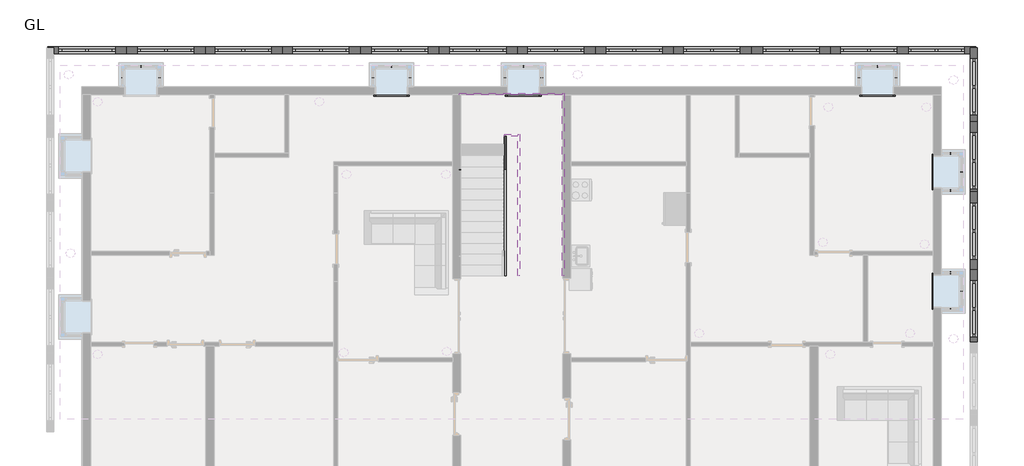
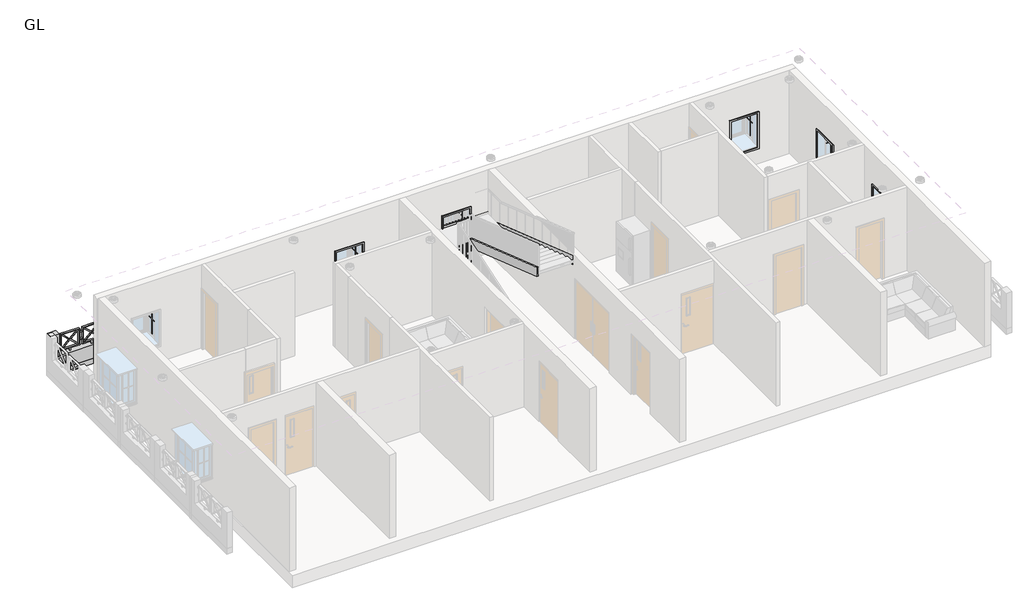
# One storey, part 5 of 5: 39 proxies, 6 members.
"""IFC4 building model written with IfcOpenShell, lengths in millimetres."""

from ifc_helpers import new_model, si_unit, frame, origin, place, context, project, spatial, polyline, outline, extrude, transform, mapped, element, save
from components import muntin_pattern_2x2_muntin_pattern_2x2_95b57395, muntin_pattern_2x2_muntin_pattern_2x2_f03ab90d, trim_window_interior_flat_picture_frame_e50cf7ae, boundary_wall_16328_150_79515850

model = new_model("IFC4")

# Units and contexts
model_context = context("Model", 3, world=origin())
ifc_project = project(units=[si_unit("LENGTHUNIT", "METRE", prefix="MILLI")], contexts=[model_context])

# Site, building, storey
site = spatial("IfcSite", under=ifc_project)
building = spatial("IfcBuilding", under=site)
storey = spatial("IfcBuildingStorey", under=building, Name="GL", Elevation=0.0)

# Proxies
placement = place(None, origin())
muntin_pattern_2x2_muntin_pattern_2x2_shape = muntin_pattern_2x2_muntin_pattern_2x2_95b57395(model_context)
element("IfcBuildingElementProxy", 1, Name="Muntin Pattern_2x2 : Muntin Pattern_2x2", ObjectType="Muntin Pattern_2x2 : Muntin Pattern_2x2", at=placement, inside=storey, context=model_context, shape_type="MappedRepresentation", body=[
    mapped(muntin_pattern_2x2_muntin_pattern_2x2_shape, transform((-10814.9987925, 8428.7317329, 730.25), x_axis=(1.0, 0.0, 0.0), y_axis=(0.0, 1.0, 0.0), z_axis=(0.0, 0.0, 1.0))),
])
element("IfcBuildingElementProxy", 2, Name="Muntin Pattern_2x2 : Muntin Pattern_2x2", ObjectType="Muntin Pattern_2x2 : Muntin Pattern_2x2", at=placement, inside=storey, context=model_context, shape_type="MappedRepresentation", body=[
    mapped(muntin_pattern_2x2_muntin_pattern_2x2_shape, transform((-3791.8987998, 8428.7317329, 730.25), x_axis=(1.0, 0.0, 0.0), y_axis=(0.0, 1.0, 0.0), z_axis=(0.0, 0.0, 1.0))),
])
element("IfcBuildingElementProxy", 3, Name="Muntin Pattern_2x2 : Muntin Pattern_2x2", ObjectType="Muntin Pattern_2x2 : Muntin Pattern_2x2", at=placement, inside=storey, context=model_context, shape_type="MappedRepresentation", body=[
    mapped(muntin_pattern_2x2_muntin_pattern_2x2_shape, transform((-96.7067989, 8428.7317329, 730.25), x_axis=(1.0, 0.0, 0.0), y_axis=(0.0, 1.0, 0.0), z_axis=(0.0, 0.0, 1.0))),
])
element("IfcBuildingElementProxy", 4, Name="Muntin Pattern_2x2 : Muntin Pattern_2x2", ObjectType="Muntin Pattern_2x2 : Muntin Pattern_2x2", at=placement, inside=storey, context=model_context, shape_type="MappedRepresentation", body=[
    mapped(muntin_pattern_2x2_muntin_pattern_2x2_shape, transform((9835.2012075, 8428.7317329, 730.25), x_axis=(1.0, 0.0, 0.0), y_axis=(0.0, 1.0, 0.0), z_axis=(0.0, 0.0, 1.0))),
])
element("IfcBuildingElementProxy", 5, Name="Muntin Pattern_2x2 : Muntin Pattern_2x2", ObjectType="Muntin Pattern_2x2 : Muntin Pattern_2x2", at=placement, inside=storey, context=model_context, shape_type="MappedRepresentation", body=[
    mapped(muntin_pattern_2x2_muntin_pattern_2x2_shape, transform((12194.2262075, 2126.3567332, 730.25), x_axis=(0.0, -1.0, 0.0), y_axis=(1.0, 0.0, 0.0), z_axis=(0.0, 0.0, 1.0))),
])
element("IfcBuildingElementProxy", 6, Name="Muntin Pattern_2x2 : Muntin Pattern_2x2", ObjectType="Muntin Pattern_2x2 : Muntin Pattern_2x2", at=placement, inside=storey, context=model_context, shape_type="MappedRepresentation", body=[
    mapped(muntin_pattern_2x2_muntin_pattern_2x2_shape, transform((12194.2262075, 5469.631733, 730.25), x_axis=(0.0, -1.0, 0.0), y_axis=(1.0, 0.0, 0.0), z_axis=(0.0, 0.0, 1.0))),
])
muntin_pattern_2x2_muntin_pattern_2x2_2_shape = muntin_pattern_2x2_muntin_pattern_2x2_f03ab90d(model_context)
element("IfcBuildingElementProxy", 7, Name="Muntin Pattern_2x2 : Muntin Pattern_2x2", ObjectType="Muntin Pattern_2x2 : Muntin Pattern_2x2", at=placement, inside=storey, context=model_context, shape_type="MappedRepresentation", body=[
    mapped(muntin_pattern_2x2_muntin_pattern_2x2_2_shape, transform((-11332.5237925, 8114.4067329, 730.25), x_axis=(0.0, -1.0, 0.0), y_axis=(1.0, 0.0, 0.0), z_axis=(0.0, 0.0, 1.0))),
])
element("IfcBuildingElementProxy", 8, Name="Muntin Pattern_2x2 : Muntin Pattern_2x2", ObjectType="Muntin Pattern_2x2 : Muntin Pattern_2x2", at=placement, inside=storey, context=model_context, shape_type="MappedRepresentation", body=[
    mapped(muntin_pattern_2x2_muntin_pattern_2x2_2_shape, transform((-10297.4737925, 8114.4067329, 730.25), x_axis=(0.0, 1.0, 0.0), y_axis=(-1.0, 0.0, 0.0), z_axis=(0.0, 0.0, 1.0))),
])
element("IfcBuildingElementProxy", 9, Name="Muntin Pattern_2x2 : Muntin Pattern_2x2", ObjectType="Muntin Pattern_2x2 : Muntin Pattern_2x2", at=placement, inside=storey, context=model_context, shape_type="MappedRepresentation", body=[
    mapped(muntin_pattern_2x2_muntin_pattern_2x2_2_shape, transform((-4309.4237998, 8114.4067329, 730.25), x_axis=(0.0, -1.0, 0.0), y_axis=(1.0, 0.0, 0.0), z_axis=(0.0, 0.0, 1.0))),
])
element("IfcBuildingElementProxy", 10, Name="Muntin Pattern_2x2 : Muntin Pattern_2x2", ObjectType="Muntin Pattern_2x2 : Muntin Pattern_2x2", at=placement, inside=storey, context=model_context, shape_type="MappedRepresentation", body=[
    mapped(muntin_pattern_2x2_muntin_pattern_2x2_2_shape, transform((-3274.3737998, 8114.4067329, 730.25), x_axis=(0.0, 1.0, 0.0), y_axis=(-1.0, 0.0, 0.0), z_axis=(0.0, 0.0, 1.0))),
])
element("IfcBuildingElementProxy", 11, Name="Muntin Pattern_2x2 : Muntin Pattern_2x2", ObjectType="Muntin Pattern_2x2 : Muntin Pattern_2x2", at=placement, inside=storey, context=model_context, shape_type="MappedRepresentation", body=[
    mapped(muntin_pattern_2x2_muntin_pattern_2x2_2_shape, transform((-614.2317989, 8114.4067329, 730.25), x_axis=(0.0, -1.0, 0.0), y_axis=(1.0, 0.0, 0.0), z_axis=(0.0, 0.0, 1.0))),
])
element("IfcBuildingElementProxy", 12, Name="Muntin Pattern_2x2 : Muntin Pattern_2x2", ObjectType="Muntin Pattern_2x2 : Muntin Pattern_2x2", at=placement, inside=storey, context=model_context, shape_type="MappedRepresentation", body=[
    mapped(muntin_pattern_2x2_muntin_pattern_2x2_2_shape, transform((420.8182011, 8114.4067329, 730.25), x_axis=(0.0, 1.0, 0.0), y_axis=(-1.0, 0.0, 0.0), z_axis=(0.0, 0.0, 1.0))),
])
element("IfcBuildingElementProxy", 13, Name="Muntin Pattern_2x2 : Muntin Pattern_2x2", ObjectType="Muntin Pattern_2x2 : Muntin Pattern_2x2", at=placement, inside=storey, context=model_context, shape_type="MappedRepresentation", body=[
    mapped(muntin_pattern_2x2_muntin_pattern_2x2_2_shape, transform((9317.6762075, 8114.4067329, 730.25), x_axis=(0.0, -1.0, 0.0), y_axis=(1.0, 0.0, 0.0), z_axis=(0.0, 0.0, 1.0))),
])
element("IfcBuildingElementProxy", 14, Name="Muntin Pattern_2x2 : Muntin Pattern_2x2", ObjectType="Muntin Pattern_2x2 : Muntin Pattern_2x2", at=placement, inside=storey, context=model_context, shape_type="MappedRepresentation", body=[
    mapped(muntin_pattern_2x2_muntin_pattern_2x2_2_shape, transform((10352.7262075, 8114.4067329, 730.25), x_axis=(0.0, 1.0, 0.0), y_axis=(-1.0, 0.0, 0.0), z_axis=(0.0, 0.0, 1.0))),
])
element("IfcBuildingElementProxy", 15, Name="Muntin Pattern_2x2 : Muntin Pattern_2x2", ObjectType="Muntin Pattern_2x2 : Muntin Pattern_2x2", at=placement, inside=storey, context=model_context, shape_type="MappedRepresentation", body=[
    mapped(muntin_pattern_2x2_muntin_pattern_2x2_2_shape, transform((11879.9012075, 2643.8817332, 730.25), x_axis=(-1.0, 0.0, 0.0), y_axis=(0.0, -1.0, 0.0), z_axis=(0.0, 0.0, 1.0))),
])
element("IfcBuildingElementProxy", 16, Name="Muntin Pattern_2x2 : Muntin Pattern_2x2", ObjectType="Muntin Pattern_2x2 : Muntin Pattern_2x2", at=placement, inside=storey, context=model_context, shape_type="MappedRepresentation", body=[
    mapped(muntin_pattern_2x2_muntin_pattern_2x2_2_shape, transform((11879.9012075, 1608.8317332, 730.25), x_axis=(1.0, 0.0, 0.0), y_axis=(0.0, 1.0, 0.0), z_axis=(0.0, 0.0, 1.0))),
])
element("IfcBuildingElementProxy", 17, Name="Muntin Pattern_2x2 : Muntin Pattern_2x2", ObjectType="Muntin Pattern_2x2 : Muntin Pattern_2x2", at=placement, inside=storey, context=model_context, shape_type="MappedRepresentation", body=[
    mapped(muntin_pattern_2x2_muntin_pattern_2x2_2_shape, transform((11879.9012075, 5987.156733, 730.25), x_axis=(-1.0, 0.0, 0.0), y_axis=(0.0, -1.0, 0.0), z_axis=(0.0, 0.0, 1.0))),
])
element("IfcBuildingElementProxy", 18, Name="Muntin Pattern_2x2 : Muntin Pattern_2x2", ObjectType="Muntin Pattern_2x2 : Muntin Pattern_2x2", at=placement, inside=storey, context=model_context, shape_type="MappedRepresentation", body=[
    mapped(muntin_pattern_2x2_muntin_pattern_2x2_2_shape, transform((11879.9012075, 4952.106733, 730.25), x_axis=(1.0, 0.0, 0.0), y_axis=(0.0, 1.0, 0.0), z_axis=(0.0, 0.0, 1.0))),
])
trim_window_interior_flat_picture_frame_shape = trim_window_interior_flat_picture_frame_e50cf7ae(model_context)
element("IfcBuildingElementProxy", 19, Name="Trim-Window-Interior-Flat : Picture Frame", ObjectType="Trim-Window-Interior-Flat : Picture Frame", at=placement, inside=storey, context=model_context, shape_type="MappedRepresentation", body=[
    mapped(trim_window_interior_flat_picture_frame_shape, transform((-3791.8987998, 7631.8067329, 1879.6), x_axis=(1.0, 0.0, 0.0), y_axis=(0.0, 0.0, 1.0), z_axis=(0.0, -1.0, 0.0))),
])
element("IfcBuildingElementProxy", 20, Name="Trim-Window-Interior-Flat : Picture Frame", ObjectType="Trim-Window-Interior-Flat : Picture Frame", at=placement, inside=storey, context=model_context, shape_type="MappedRepresentation", body=[
    mapped(trim_window_interior_flat_picture_frame_shape, transform((-96.7067989, 7631.8067329, 1879.6), x_axis=(1.0, 0.0, 0.0), y_axis=(0.0, 0.0, 1.0), z_axis=(0.0, -1.0, 0.0))),
])
element("IfcBuildingElementProxy", 21, Name="Trim-Window-Interior-Flat : Picture Frame", ObjectType="Trim-Window-Interior-Flat : Picture Frame", at=placement, inside=storey, context=model_context, shape_type="MappedRepresentation", body=[
    mapped(trim_window_interior_flat_picture_frame_shape, transform((9835.2012075, 7631.8067329, 1879.6), x_axis=(1.0, 0.0, 0.0), y_axis=(0.0, 0.0, 1.0), z_axis=(0.0, -1.0, 0.0))),
])
element("IfcBuildingElementProxy", 22, Name="Trim-Window-Interior-Flat : Picture Frame", ObjectType="Trim-Window-Interior-Flat : Picture Frame", at=placement, inside=storey, context=model_context, shape_type="MappedRepresentation", body=[
    mapped(trim_window_interior_flat_picture_frame_shape, transform((11397.3012075, 2126.3567332, 1879.6), x_axis=(0.0, -1.0, 0.0), y_axis=(0.0, 0.0, 1.0), z_axis=(-1.0, 0.0, 0.0))),
])
element("IfcBuildingElementProxy", 23, Name="Trim-Window-Interior-Flat : Picture Frame", ObjectType="Trim-Window-Interior-Flat : Picture Frame", at=placement, inside=storey, context=model_context, shape_type="MappedRepresentation", body=[
    mapped(trim_window_interior_flat_picture_frame_shape, transform((11397.3012075, 5469.631733, 1879.6), x_axis=(0.0, -1.0, 0.0), y_axis=(0.0, 0.0, 1.0), z_axis=(-1.0, 0.0, 0.0))),
])
boundary_wall_16328_150_shape = boundary_wall_16328_150_79515850(model_context)
element("IfcBuildingElementProxy", 24, Name="boundary_wall__16328 : 150", ObjectType="boundary_wall__16328 : 150", at=placement, inside=storey, context=model_context, shape_type="MappedRepresentation", body=[
    mapped(boundary_wall_16328_150_shape, transform((-12332.6487992, 8889.1067339, 0.0), x_axis=(1.0, 0.0, 0.0), y_axis=(0.0, 1.0, 0.0), z_axis=(0.0, 0.0, 1.0))),
])
element("IfcBuildingElementProxy", 25, Name="boundary_wall__16328 : 150", ObjectType="boundary_wall__16328 : 150", at=placement, inside=storey, context=model_context, shape_type="MappedRepresentation", body=[
    mapped(boundary_wall_16328_150_shape, transform((-10122.8487992, 8889.1067339, 0.0), x_axis=(1.0, 0.0, 0.0), y_axis=(0.0, 1.0, 0.0), z_axis=(0.0, 0.0, 1.0))),
])
element("IfcBuildingElementProxy", 26, Name="boundary_wall__16328 : 150", ObjectType="boundary_wall__16328 : 150", at=placement, inside=storey, context=model_context, shape_type="MappedRepresentation", body=[
    mapped(boundary_wall_16328_150_shape, transform((-7951.1487994, 8889.1067339, 0.0), x_axis=(1.0, 0.0, 0.0), y_axis=(0.0, 1.0, 0.0), z_axis=(0.0, 0.0, 1.0))),
])
element("IfcBuildingElementProxy", 27, Name="boundary_wall__16328 : 150", ObjectType="boundary_wall__16328 : 150", at=placement, inside=storey, context=model_context, shape_type="MappedRepresentation", body=[
    mapped(boundary_wall_16328_150_shape, transform((-5773.0987998, 8889.1067339, 0.0), x_axis=(1.0, 0.0, 0.0), y_axis=(0.0, 1.0, 0.0), z_axis=(0.0, 0.0, 1.0))),
])
element("IfcBuildingElementProxy", 28, Name="boundary_wall__16328 : 150", ObjectType="boundary_wall__16328 : 150", at=placement, inside=storey, context=model_context, shape_type="MappedRepresentation", body=[
    mapped(boundary_wall_16328_150_shape, transform((-3563.2987998, 8889.1067339, 0.0), x_axis=(1.0, 0.0, 0.0), y_axis=(0.0, 1.0, 0.0), z_axis=(0.0, 0.0, 1.0))),
])
element("IfcBuildingElementProxy", 29, Name="boundary_wall__16328 : 150", ObjectType="boundary_wall__16328 : 150", at=placement, inside=storey, context=model_context, shape_type="MappedRepresentation", body=[
    mapped(boundary_wall_16328_150_shape, transform((-1366.7067989, 8889.1067339, 0.0), x_axis=(1.0, 0.0, 0.0), y_axis=(0.0, 1.0, 0.0), z_axis=(0.0, 0.0, 1.0))),
])
element("IfcBuildingElementProxy", 30, Name="boundary_wall__16328 : 150", ObjectType="boundary_wall__16328 : 150", at=placement, inside=storey, context=model_context, shape_type="MappedRepresentation", body=[
    mapped(boundary_wall_16328_150_shape, transform((817.6932011, 8889.1067339, 0.0), x_axis=(1.0, 0.0, 0.0), y_axis=(0.0, 1.0, 0.0), z_axis=(0.0, 0.0, 1.0))),
])
element("IfcBuildingElementProxy", 31, Name="boundary_wall__16328 : 150", ObjectType="boundary_wall__16328 : 150", at=placement, inside=storey, context=model_context, shape_type="MappedRepresentation", body=[
    mapped(boundary_wall_16328_150_shape, transform((3015.3012075, 8889.1067339, 0.0), x_axis=(1.0, 0.0, 0.0), y_axis=(0.0, 1.0, 0.0), z_axis=(0.0, 0.0, 1.0))),
])
element("IfcBuildingElementProxy", 32, Name="boundary_wall__16328 : 150", ObjectType="boundary_wall__16328 : 150", at=placement, inside=storey, context=model_context, shape_type="MappedRepresentation", body=[
    mapped(boundary_wall_16328_150_shape, transform((5193.351208, 8889.1067339, 0.0), x_axis=(1.0, 0.0, 0.0), y_axis=(0.0, 1.0, 0.0), z_axis=(0.0, 0.0, 1.0))),
])
element("IfcBuildingElementProxy", 33, Name="boundary_wall__16328 : 150", ObjectType="boundary_wall__16328 : 150", at=placement, inside=storey, context=model_context, shape_type="MappedRepresentation", body=[
    mapped(boundary_wall_16328_150_shape, transform((7415.8512079, 8889.1067339, 0.0), x_axis=(1.0, 0.0, 0.0), y_axis=(0.0, 1.0, 0.0), z_axis=(0.0, 0.0, 1.0))),
])
element("IfcBuildingElementProxy", 34, Name="boundary_wall__16328 : 150", ObjectType="boundary_wall__16328 : 150", at=placement, inside=storey, context=model_context, shape_type="MappedRepresentation", body=[
    mapped(boundary_wall_16328_150_shape, transform((9593.9012075, 8889.1067339, 0.0), x_axis=(1.0, 0.0, 0.0), y_axis=(0.0, 1.0, 0.0), z_axis=(0.0, 0.0, 1.0))),
])
element("IfcBuildingElementProxy", 35, Name="boundary_wall__16328 : 150", ObjectType="boundary_wall__16328 : 150", at=placement, inside=storey, context=model_context, shape_type="MappedRepresentation", body=[
    mapped(boundary_wall_16328_150_shape, transform((11486.2012075, 8889.1067339, 0.0), x_axis=(1.0, 0.0, 0.0), y_axis=(0.0, 1.0, 0.0), z_axis=(0.0, 0.0, 1.0))),
])
element("IfcBuildingElementProxy", 36, Name="boundary_wall__16328 : 150", ObjectType="boundary_wall__16328 : 150", at=placement, inside=storey, context=model_context, shape_type="MappedRepresentation", body=[
    mapped(boundary_wall_16328_150_shape, transform((12540.3012043, 7860.4067329, 0.0), x_axis=(0.0, 1.0, 0.0), y_axis=(-1.0, 0.0, 0.0), z_axis=(0.0, 0.0, 1.0))),
])
element("IfcBuildingElementProxy", 37, Name="boundary_wall__16328 : 150", ObjectType="boundary_wall__16328 : 150", at=placement, inside=storey, context=model_context, shape_type="MappedRepresentation", body=[
    mapped(boundary_wall_16328_150_shape, transform((12540.3012043, 5783.9567329, 0.0), x_axis=(0.0, 1.0, 0.0), y_axis=(-1.0, 0.0, 0.0), z_axis=(0.0, 0.0, 1.0))),
])
element("IfcBuildingElementProxy", 38, Name="boundary_wall__16328 : 150", ObjectType="boundary_wall__16328 : 150", at=placement, inside=storey, context=model_context, shape_type="MappedRepresentation", body=[
    mapped(boundary_wall_16328_150_shape, transform((12540.3012043, 3815.040939, 0.0), x_axis=(0.0, 1.0, 0.0), y_axis=(-1.0, 0.0, 0.0), z_axis=(0.0, 0.0, 1.0))),
])
element("IfcBuildingElementProxy", 39, Name="boundary_wall__16328 : 150", ObjectType="boundary_wall__16328 : 150", at=placement, inside=storey, context=model_context, shape_type="MappedRepresentation", body=[
    mapped(boundary_wall_16328_150_shape, transform((12540.3012043, 1631.0567332, 0.0), x_axis=(0.0, 1.0, 0.0), y_axis=(-1.0, 0.0, 0.0), z_axis=(0.0, 0.0, 1.0))),
])

# Members
element("IfcMember", 40, ObjectType="Stringer - 2\" Width", at=placement, inside=storey, context=model_context, shape_type="SweptSolid", body=[
    extrude(outline(polyline([(2564.5067329, 0.0), (2564.5067329, 193.238056), (6486.7524627, 1524.0), (7435.4093802, 1524.0), (2943.6199065, 0.0), (2564.5067329, 0.0)])), frame((-1899.5987998, 0.0, 0.0), z_axis=(1.0, 0.0, 0.0), x_axis=(0.0, 1.0, 0.0)), (0.0, 0.0, 1.0), 50.8),
])
element("IfcMember", 41, ObjectType="Stringer - 2\" Width", at=placement, inside=storey, context=model_context, shape_type="SweptSolid", body=[
    extrude(outline(polyline([(-1899.5987998, 7631.8067329), (-1899.5987998, 7682.6067329), (996.0012002, 7682.6067329), (996.0012002, 7631.8067329), (-1899.5987998, 7631.8067329)])), frame((0.0, 0.0, 1219.2), z_axis=(0.0, 0.0, 1.0), x_axis=(1.0, 0.0, 0.0)), (0.0, 0.0, 1.0), 304.8),
])
element("IfcMember", 42, ObjectType="Stringer - 2\" Width", at=placement, inside=storey, context=model_context, shape_type="SweptSolid", body=[
    extrude(outline(polyline([(7682.6067329, 1248.925556), (7682.6067329, 1219.2), (6821.5619804, 1219.2), (2564.5067329, 2663.5580304), (2564.5067329, 2985.4237702), (7682.6067329, 1248.925556)])), frame((996.0012002, 0.0, 0.0), z_axis=(1.0, 0.0, 0.0), x_axis=(0.0, 1.0, 0.0)), (0.0, 0.0, 1.0), 50.8),
])
element("IfcMember", 43, ObjectType="Stringer - 2\" Width", at=placement, inside=storey, context=model_context, shape_type="SweptSolid", body=[
    extrude(outline(polyline([(2564.5067329, 0.0), (2564.5067329, 193.238056), (6476.1067329, 1520.388056), (6476.1067329, 1198.5223161), (2943.6199065, 0.0), (2564.5067329, 0.0)])), frame((-629.5987998, 0.0, 0.0), z_axis=(1.0, 0.0, 0.0), x_axis=(0.0, 1.0, 0.0)), (0.0, 0.0, 1.0), 50.8),
])
element("IfcMember", 44, ObjectType="Stringer - 2\" Width", at=placement, inside=storey, context=model_context, shape_type="SweptSolid", body=[
    extrude(outline(polyline([(-629.5987998, 6476.1067329), (-629.5987998, 6526.9067329), (-248.5987915, 6526.9067329), (-248.5987915, 6476.1067329), (-629.5987998, 6476.1067329)])), frame((0.0, 0.0, 1219.2), z_axis=(0.0, 0.0, 1.0), x_axis=(1.0, 0.0, 0.0)), (0.0, 0.0, 1.0), 304.8),
])
element("IfcMember", 45, ObjectType="Stringer - 2\" Width", at=placement, inside=storey, context=model_context, shape_type="SweptSolid", body=[
    extrude(outline(polyline([(6526.9067329, 1641.038056), (6526.9067329, 1319.1723161), (2564.5067329, 2663.5580304), (2564.5067329, 2985.4237702), (6526.9067329, 1641.038056)])), frame((-248.5987915, 0.0, 0.0), z_axis=(1.0, 0.0, 0.0), x_axis=(0.0, 1.0, 0.0)), (0.0, 0.0, 1.0), 50.8),
])

save(model, "model.ifc")

# Revit data of these elements
# Type "Muntin Pattern_2x2 : Muntin Pattern_2x2"
#   Width [instance default] = 4' - 0"
#   Thickness = 0' - 0 1/2"
#   Height [instance default] = 4' - 0"
#   Distance = 0' - 0 3/4"
#   Interior Material [instance default] = none
#   Exterior Material [instance default] = none
#   Default Elevation = 0
# Type "Trim-Window-Interior-Flat : Picture Frame"
#   Trim Thickness_Picture Frame = 0' - 1 1/4"
#   Trim Width = 0' - 2 1/4"
#   Trim Thickness_with Sill = 0' - 0 3/4"
#   Sill Thickness = 0' - 1 1/4"
#   Opening Width [instance default] = 2' - 0"
#   Opening Height [instance default] = 3' - 0"
#   Default Elevation = 4' - 0"
#   Sill = no
#   Picture Frame = yes
#   Trim Material [instance default] = none
# Type "boundary_wall__16328 : 150"
#   Wight Hand 2 = 0' - 11.81102"
#   Wight Hand 1 = 0' - 11.81102"
#   Void Wight = 5' - 2.99213"
#   Top.High = 2' - 7.49606"
#   F.base = 0' - 3.93701"
#   F.Wight 2 = 2' - 1.59055"
#   F.Wight 1 = 2' - 1.59055"
#   F.R = 0' - 3.93701"
#   F.L = 0' - 3.93701"
#   F.High = 1' - 11.62205"
#   Bace.High = 1' - 7.68504"
#   Default Elevation = 0
# Elements 1, 2, 3, 4, 5, 6 (IfcBuildingElementProxy, "Muntin Pattern_2x2 : Muntin Pattern_2x2")
#   Width = 2' - 6 1/2"
#   Height = 3' - 6 1/2"
#   Interior Material = Wood - Stained
#   Exterior Material = Clad - White
#   Phase Created = New Construction
#   Materials on its faces: "Clad - White", "Wood - Stained"
# Elements 7, 8, 9, 10, 11, 12, 13, 14, 15, 16, 17, 18 (IfcBuildingElementProxy, "Muntin Pattern_2x2 : Muntin Pattern_2x2")
#   Width = 1' - 2 1/2"
#   Height = 3' - 6 1/2"
#   Interior Material = Wood - Stained
#   Exterior Material = Clad - White
#   Phase Created = New Construction
#   Materials on its faces: "Clad - White", "Wood - Stained"
# Elements 19, 20, 21, 22, 23 (IfcBuildingElementProxy, "Trim-Window-Interior-Flat : Picture Frame")
#   Opening Width = 3' - 0"
#   Opening Height = 4' - 2"
#   Trim Material = Wood - Stained
#   Phase Created = New Construction
#   Materials on its faces: "Wood - Stained"
# Elements 24, 25, 26, 27, 28, 29, 30, 31, 32, 33, 34, 35, 36, 37, 38, 39 (IfcBuildingElementProxy, "boundary_wall__16328 : 150")
#   Phase Created = New Construction
#   Materials on its faces: "Metal"
# Elements 40, 41, 42, 43, 44, 45 (IfcMember, "Stringer - 2\" Width")
#   Phase Created = New Construction
# Materials
#   "Clad - White": class "Wood", colour RGB 242 242 238, transparency 0, Cost = 0
#   "Wood - Stained": class "Wood", colour RGB 224 178 126, transparency 0, Cost = 0
#   "Metal": class "Generic", colour RGB 65 64 62, transparency 0, Cost = 0
